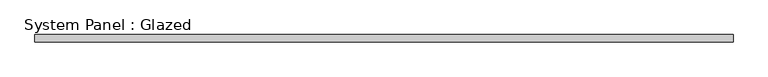
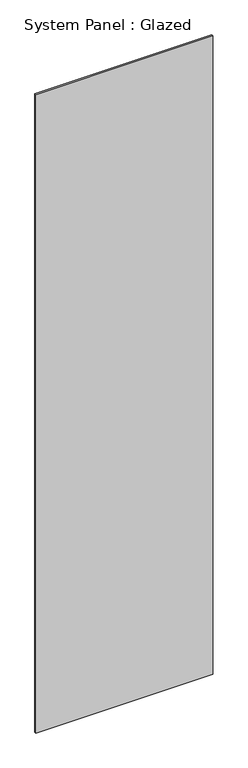
"""IFC4 building model written with IfcOpenShell, lengths in millimetres: plate geometry, System Panel : Glazed."""

from ifc_helpers import new_model, si_unit, origin, origin_with_axes, place, context, project, spatial, polyline, outline, extrude, source, transform, mapped, element, save


def system_panel_glazed_b4ce2d81(model_context):
    return source(origin(), model_context, "Body", "SweptSolid", [
        extrude(outline(polyline([(1238.25, 19.05), (-1238.25, 19.05), (-1238.25, 44.45), (1238.25, 44.45), (1238.25, 19.05)])), origin_with_axes(), (0.0, 0.0, 1.0), 9448.8),
    ])


if __name__ == "__main__":
    model = new_model("IFC4")
    model_context = context("Model", 3, world=origin())
    ifc_project = project(units=[si_unit("LENGTHUNIT", "METRE", prefix="MILLI")], contexts=[model_context])
    site = spatial("IfcSite", under=ifc_project)
    building = spatial("IfcBuilding", under=site)
    placement = place(None, origin())
    system_panel_glazed_shape = system_panel_glazed_b4ce2d81(model_context)
    element("IfcPlate", 1, ObjectType="System Panel : Glazed", at=placement, inside=building, context=model_context, shape_type="MappedRepresentation", body=[
        mapped(system_panel_glazed_shape, transform((0.0, 0.0, 0.0), x_axis=(1.0, 0.0, 0.0), y_axis=(0.0, 1.0, 0.0), z_axis=(0.0, 0.0, 1.0))),
    ])
    save(model, "model.ifc")

# Revit data of these elements
# Type "System Panel : Glazed"
#   Construction Type Id = "GSP4R"
#   Analytic Construction = "1/8 in Pilkington single glazing"
#   Visual Light Transmittance = 0.9
#   Solar Heat Gain Coefficient = 0.86
#   Heat Transfer Coefficient (U) = 1.18115 BTU/(h·ft²·°F)
#   Define Thermal Properties by = 1
# Element 1 (IfcPlate, "System Panel : Glazed")
#   Materials on its faces: "Glass"
# Materials
#   "Glass": class "Glass", colour RGB 0 128 192, transparency 0.75, Description = "Soda Lime Glass", Cost = 0
